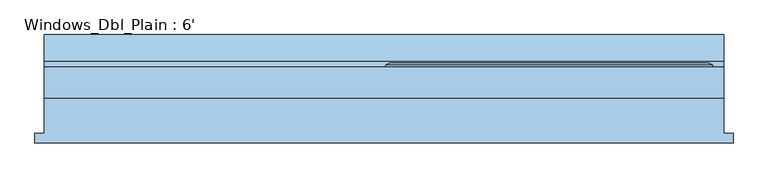
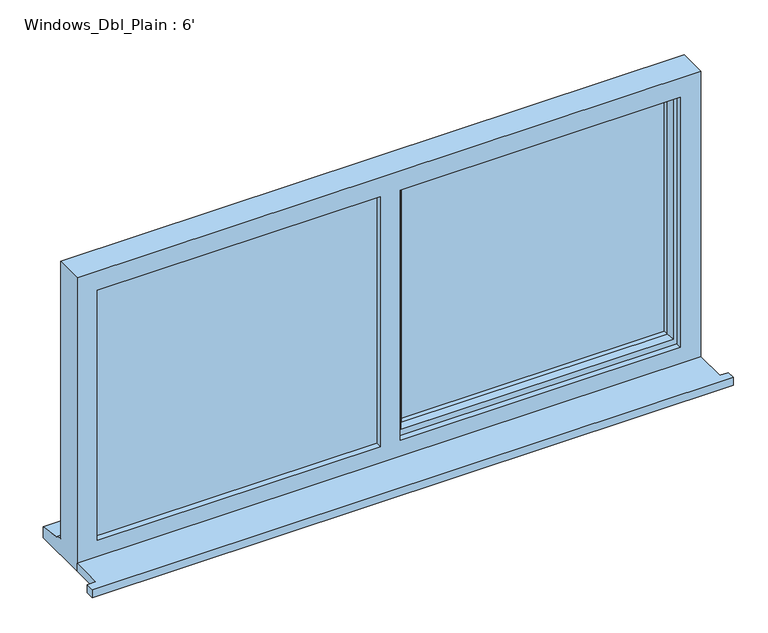
"""IFC4 building model written with IfcOpenShell, lengths in millimetres: window geometry, Windows_Dbl_Plain : 6'."""

from ifc_helpers import new_model, si_unit, frame, origin, place, context, project, spatial, polyline, outline, extrude, faceted_brep, source, transform, mapped, element, save


def windows_dbl_plain_6_22e4277a(model_context):
    return source(origin(), model_context, "Body", "SolidModel", [
        extrude(outline(polyline([(-1224.4, -130.8434322), (-1224.4, -105.8434322), (-1199.4, -105.8434322), (-1199.4, -10.2434322), (629.4, -10.2434322), (629.4, -105.8434322), (654.4, -105.8434322), (654.4, -130.8434322), (-1224.4, -130.8434322)])), frame((0.0, 0.0, 1200.0), z_axis=(0.0, 0.0, 1.0), x_axis=(1.0, 0.0, 0.0)), (0.0, 0.0, 1.0), 25.0),
        faceted_brep([(-280.0, 72.7565678, 2080.0), (-280.0, 78.5300705, 2080.0), (-280.0, 78.5300705, 1253.0), (-280.0, 72.7565678, 1253.0), (-270.0, 7.7565678, 2070.0), (-270.0, 72.7565678, 2070.0), (-270.0, 72.7565678, 1263.0), (-270.0, 7.7565678, 1263.0), (-230.0, 22.2494677, 2030.0), (-240.1480377, 7.7565678, 2040.1480377), (-240.1480377, 7.7565678, 1292.8519623), (-230.0, 22.2494677, 1303.0), (-230.0, 36.7565678, 2030.0), (-230.0, 36.7565678, 1303.0), (-240.0, 60.7565678, 2040.0), (-240.0, 36.7565678, 2040.0), (-240.0, 36.7565678, 1293.0), (-240.0, 60.7565678, 1293.0), (-230.0, 78.5300705, 2030.0), (-230.0, 60.7565678, 2030.0), (-230.0, 60.7565678, 1303.0), (-230.0, 78.5300705, 1303.0), (-247.4457548, 84.3035732, 2047.4457548), (-247.4457548, 84.3035732, 1285.5542452), (-269.2153903, 84.3035732, 2069.2153903), (-269.2153903, 84.3035732, 1263.7846097), (599.4, 78.5300705, 1253.0), (599.4, 72.7565678, 1253.0), (589.4, 72.7565678, 1263.0), (589.4, 7.7565678, 1263.0), (559.5480377, 7.7565678, 1292.8519623), (549.4, 22.2494677, 1303.0), (549.4, 36.7565678, 1303.0), (559.4, 36.7565678, 1293.0), (559.4, 60.7565678, 1293.0), (549.4, 60.7565678, 1303.0), (549.4, 78.5300705, 1303.0), (566.8457548, 84.3035732, 1285.5542452), (588.6153903, 84.3035732, 1263.7846097), (599.4, 78.5300705, 2080.0), (599.4, 72.7565678, 2080.0), (589.4, 72.7565678, 2070.0), (589.4, 7.7565678, 2070.0), (559.5480377, 7.7565678, 2040.1480377), (549.4, 22.2494677, 2030.0), (549.4, 36.7565678, 2030.0), (559.4, 36.7565678, 2040.0), (559.4, 60.7565678, 2040.0), (549.4, 60.7565678, 2030.0), (549.4, 78.5300705, 2030.0), (566.8457548, 84.3035732, 2047.4457548), (588.6153903, 84.3035732, 2069.2153903)], [[[0, 1, 2, 3]], [[4, 5, 6, 7]], [[8, 9, 10, 11]], [[12, 8, 11, 13]], [[14, 15, 16, 17]], [[18, 19, 20, 21]], [[22, 18, 21, 23]], [[1, 24, 25, 2]], [[3, 2, 26, 27]], [[7, 6, 28, 29]], [[11, 10, 30, 31]], [[13, 11, 31, 32]], [[17, 16, 33, 34]], [[21, 20, 35, 36]], [[23, 21, 36, 37]], [[2, 25, 38, 26]], [[27, 26, 39, 40]], [[29, 28, 41, 42]], [[31, 30, 43, 44]], [[32, 31, 44, 45]], [[34, 33, 46, 47]], [[36, 35, 48, 49]], [[37, 36, 49, 50]], [[26, 38, 51, 39]], [[40, 39, 1, 0]], [[3, 27, 40, 0], [5, 41, 28, 6]], [[42, 41, 5, 4]], [[7, 29, 42, 4], [9, 43, 30, 10]], [[44, 43, 9, 8]], [[45, 44, 8, 12]], [[15, 46, 33, 16], [13, 32, 45, 12]], [[47, 46, 15, 14]], [[17, 34, 47, 14], [19, 48, 35, 20]], [[49, 48, 19, 18]], [[50, 49, 18, 22]], [[24, 51, 38, 25], [23, 37, 50, 22]], [[39, 51, 24, 1]]]),
        extrude(outline(polyline([(2050.0, -310.0), (2070.0, -310.0), (2070.0, -1159.4), (1263.0, -1159.4), (1263.0, -310.0), (1283.0, -310.0), (1283.0, -1139.4), (2050.0, -1139.4), (2050.0, -310.0)])), frame((0.0, 31.7565678, 0.0), z_axis=(0.0, 1.0, 0.0), x_axis=(0.0, 0.0, 1.0)), (0.0, 0.0, 1.0), 41.0),
        faceted_brep([(629.4, -10.2434322, 2110.0), (-1199.4, -10.2434322, 2110.0), (-1199.4, -10.2434322, 1200.0), (629.4, -10.2434322, 1200.0), (569.4, -10.2434322, 2050.0), (569.4, -10.2434322, 1275.0), (-252.0, -10.2434322, 1275.0), (-252.0, -10.2434322, 2050.0), (-310.0, -10.2434322, 2050.0), (-310.0, -10.2434322, 1275.0), (-1139.4, -10.2434322, 1275.0), (-1139.4, -10.2434322, 2050.0), (-1199.4, 72.7565678, 2110.0), (-1199.4, 72.7565678, 1251.0), (-1199.4, 87.7565678, 1249.68767), (-1199.4, 87.7565678, 1244.7449676), (-1199.4, 160.2565678, 1233.8088847), (-1199.4, 160.2565678, 1200.0), (629.4, 72.7565678, 2110.0), (629.4, 72.7565678, 1251.0), (-1159.4, 72.7565678, 2070.0), (-1159.4, 72.7565678, 1263.0), (-310.0, 72.7565678, 1263.0), (-310.0, 72.7565678, 2070.0), (-270.0, 72.7565678, 2070.0), (-270.0, 72.7565678, 1263.0), (589.4, 72.7565678, 1263.0), (589.4, 72.7565678, 2070.0), (-1159.4, 7.7565678, 2070.0), (-1159.4, 7.7565678, 1263.0), (-300.0, 7.7565678, 2070.0), (-300.0, 7.7565678, 1263.0), (-310.0, 7.7565678, 2050.0), (-1139.4, 7.7565678, 2050.0), (-1139.4, 7.7565678, 1275.0), (-310.0, 7.7565678, 1275.0), (-270.0, 7.7565678, 2070.0), (589.4, 7.7565678, 2070.0), (589.4, 7.7565678, 1263.0), (-270.0, 7.7565678, 1263.0), (569.4, 7.7565678, 2050.0), (-252.0, 7.7565678, 2050.0), (-252.0, 7.7565678, 1275.0), (569.4, 7.7565678, 1275.0), (-310.0, 31.7565678, 2070.0), (-300.0, 31.7565678, 2070.0), (629.4, 160.2565678, 1200.0), (629.4, 160.2565678, 1233.8088847), (629.4, 87.7565678, 1244.7449676), (629.4, 87.7565678, 1249.68767), (-300.0, 31.7565678, 1263.0), (-310.0, 31.7565678, 1263.0)], [[[0, 1, 2, 3], [4, 5, 6, 7], [8, 9, 10, 11]], [[2, 1, 12, 13, 14, 15, 16, 17]], [[13, 12, 18, 19], [20, 21, 22, 23], [24, 25, 26, 27]], [[21, 20, 28, 29]], [[28, 30, 31, 29], [32, 33, 34, 35]], [[36, 37, 38, 39], [40, 41, 42, 43]], [[33, 11, 10, 34]], [[1, 0, 18, 12]], [[28, 20, 23, 44, 45, 30]], [[27, 37, 36, 24]], [[11, 33, 32, 8]], [[40, 4, 7, 41]], [[19, 18, 0, 3, 46, 47, 48, 49]], [[27, 26, 38, 37]], [[4, 40, 43, 5]], [[45, 50, 31, 30]], [[50, 45, 44, 51]], [[51, 44, 23, 22]], [[25, 24, 36, 39]], [[41, 7, 6, 42]], [[8, 32, 35, 9]], [[46, 3, 2, 17]], [[47, 46, 17, 16]], [[48, 47, 16, 15]], [[49, 48, 15, 14]], [[19, 49, 14, 13]], [[22, 21, 29, 31, 50, 51]], [[26, 25, 39, 38]], [[6, 5, 43, 42]], [[35, 34, 10, 9]]]),
        extrude(outline(polyline([(-1159.4, 31.7565678), (-300.0, 31.7565678), (-300.0, 7.7565678), (-1159.4, 7.7565678), (-1159.4, 31.7565678)])), frame((0.0, 0.0, 1263.0), z_axis=(0.0, 0.0, 1.0), x_axis=(1.0, 0.0, 0.0)), (0.0, 0.0, 1.0), 807.0),
        extrude(outline(polyline([(559.4, 36.7565678), (-240.0, 36.7565678), (-240.0, 60.7565678), (559.4, 60.7565678), (559.4, 36.7565678)])), frame((0.0, 0.0, 1293.0), z_axis=(0.0, 0.0, 1.0), x_axis=(1.0, 0.0, 0.0)), (0.0, 0.0, 1.0), 747.0),
    ])


if __name__ == "__main__":
    model = new_model("IFC4")
    model_context = context("Model", 3, world=origin())
    ifc_project = project(units=[si_unit("LENGTHUNIT", "METRE", prefix="MILLI")], contexts=[model_context])
    site = spatial("IfcSite", under=ifc_project)
    building = spatial("IfcBuilding", under=site)
    placement = place(None, origin())
    windows_dbl_plain_6_shape = windows_dbl_plain_6_22e4277a(model_context)
    element("IfcWindow", 1, ObjectType="Windows_Dbl_Plain : 6'", at=placement, inside=building, context=model_context, shape_type="MappedRepresentation", body=[
        mapped(windows_dbl_plain_6_shape, transform((0.0, 0.0, 0.0), x_axis=(1.0, 0.0, 0.0), y_axis=(0.0, 1.0, 0.0), z_axis=(0.0, 0.0, 1.0))),
    ])
    save(model, "model.ifc")

# Revit data of these elements
# Type "Windows_Dbl_Plain : 6'"
#   Type Mark = "62"
#   Operation = "DoublePanelVertical"
#   Construction Type Id = "GSP4R"
#   Manufacturer = "Revit"
#   Keynote = "L10"
#   Analytic Construction = "1/8 in Pilkington single glazing"
#   Wrap Layers (Ext) from Ext = 0.336286 ft
#   Wrap Layers (Int) from Ext = 0.582349 ft
#   Window Board Projection = 0.082021 ft
#   Window Board Extension = 0.082021 ft
#   Visual Light Transmittance = 0.9
#   Solar Heat Gain Coefficient = 0.78
#   Rough Width = 6.0 ft
#   Rough Height = 2.985564 ft
#   Height = 2.985564 ft
#   Width = 6.0 ft
#   Heat Transfer Coefficient (U) = 3.6886 W/(m²·K)
#   Glazing Thickness = 0.07874 ft
#   FrameOffset - External = 0.164042 ft
#   Frame Depth = 0.213255 ft
#   Default Head Height = 6.922572 ft
#   Cill Depth = 0.287073 ft
#   Cavity Closer Width = 0.164042 ft
#   Cavity Closer Offset from Ext = 0.336286 ft
#   Cavity Closer Depth = 0.278871 ft
#   Vis - Cavity Closers = yes
#   Define Thermal Properties by = 1
#   Material Trim = Window Frame
#   Material Glass = Glass
#   Material Frame = Window Frame
#   Wall Closure = (empty or 0)
# Element 1 (IfcWindow, "Windows_Dbl_Plain : 6'")
#   Materials on its faces: "Window Frame", "Glass"
# Materials
#   "Window Frame": colour RGB 249 249 249, transparency 0, Keynote = "L10", Cost = 0
#   "Glass": class "Glass", colour RGB 0 128 192, transparency 0.9, Description = "Soda Lime Glass", Cost = 0
